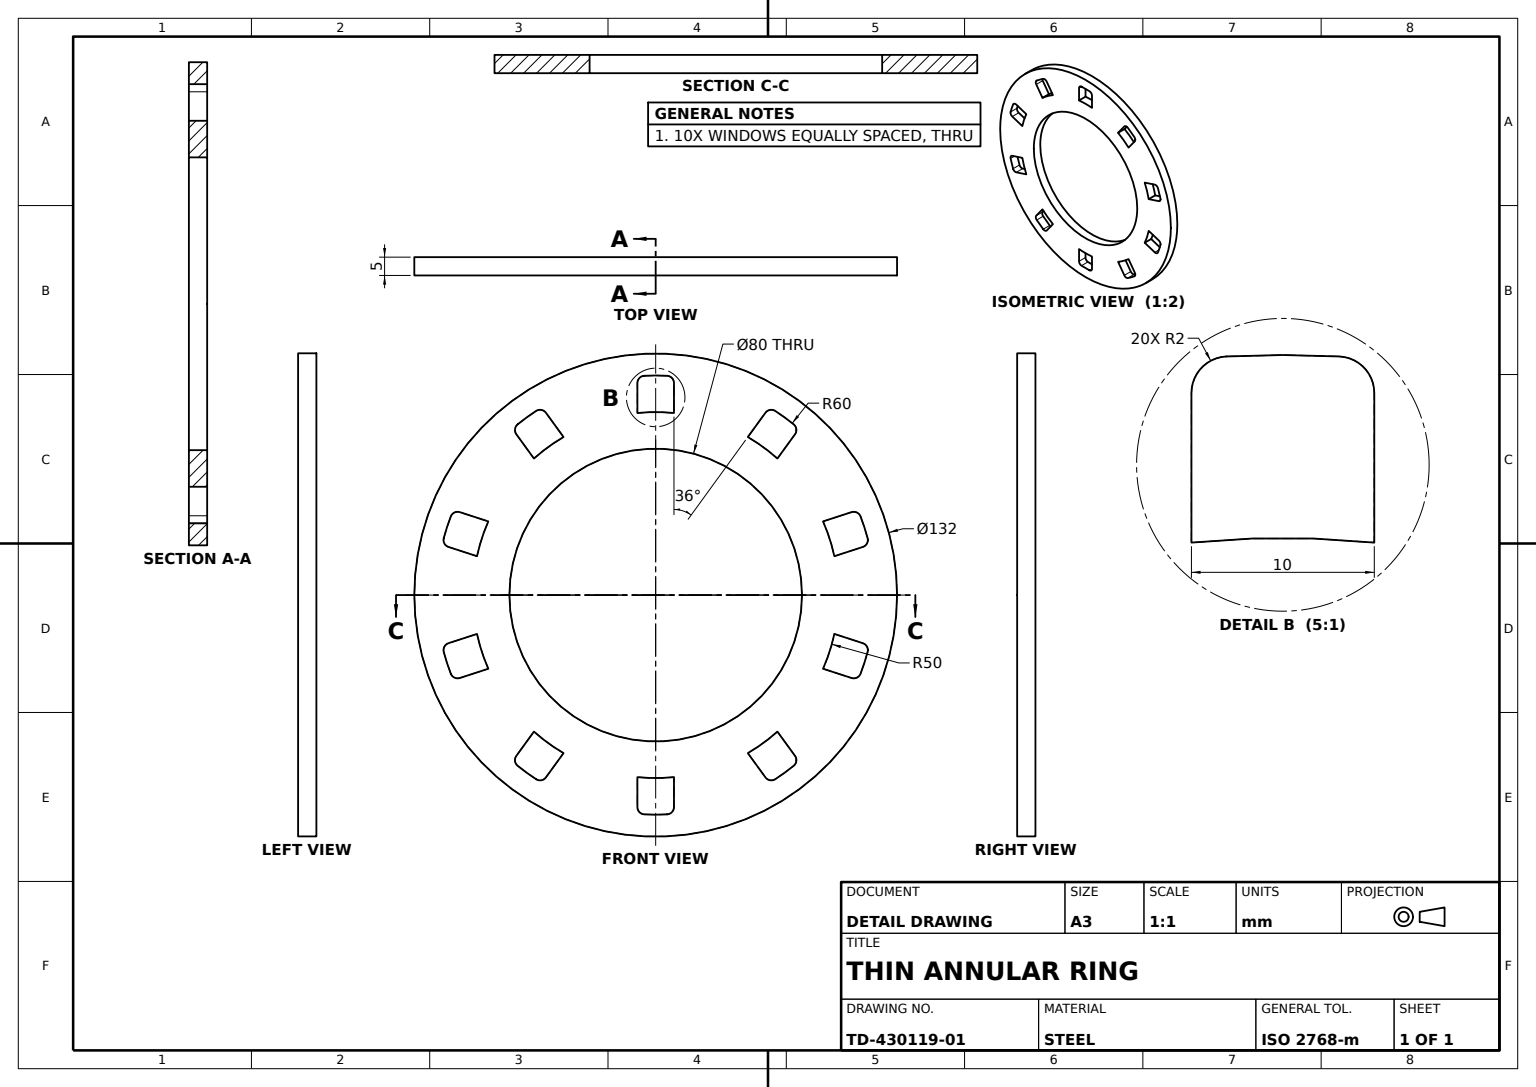
from build123d import *

# Parameters (mm, degrees)
RING_OUTLINE_SKETCH_132_R = 66
RING_DISC_132X5_DEPTH     = 5
WINDOW_CUT_DEPTH          = 25
WINDOW_PATTERN_10X_COUNT  = 10
BORE_SKETCH_80_R          = 40
CENTRE_BORE_80_DEPTH      = 25


with BuildPart() as part:
    # Ring Outline Sketch Ø132 → Ring Disc Ø132x5 (new body)
    with BuildSketch(Plane.XY):
        Circle(RING_OUTLINE_SKETCH_132_R)
    extrude(amount=RING_DISC_132X5_DEPTH)

    # Window Sketch → Window Cut (cut)
    with BuildSketch(Plane.XY.offset(5)):
        with BuildLine():
            Line((5, 49.749371855), (5, 57.92236183))
            ThreePointArc((5, 57.92236183), (4.450326955, 59.299515316), (3.103448276, 59.919684652))
            ThreePointArc((3.103448276, 59.919684652), (0, 60), (-3.103448276, 59.919684652))
            ThreePointArc((-3.103448276, 59.919684652), (-4.450326955, 59.299515316), (-5, 57.92236183))
            Line((-5, 57.92236183), (-5, 49.749371855))
            ThreePointArc((-5, 49.749371855), (0, 50), (5, 49.749371855))
        make_face()
    window_cut = extrude(amount=-WINDOW_CUT_DEPTH, mode=Mode.SUBTRACT)

    # Window Pattern 10x: Window Cut ×10 about axis
    window_pattern_10x_axis = Axis((0, 0, 0), (0, 0, 1))
    for i in range(1, WINDOW_PATTERN_10X_COUNT):
        add(window_cut.rotate(window_pattern_10x_axis, i * 360 / WINDOW_PATTERN_10X_COUNT), mode=Mode.SUBTRACT)

    # Bore Sketch Ø80 → Centre Bore Ø80 (cut)
    with BuildSketch(Plane.XY.offset(5)):
        Circle(BORE_SKETCH_80_R)
    extrude(amount=-CENTRE_BORE_80_DEPTH, mode=Mode.SUBTRACT)


solid = part.part
